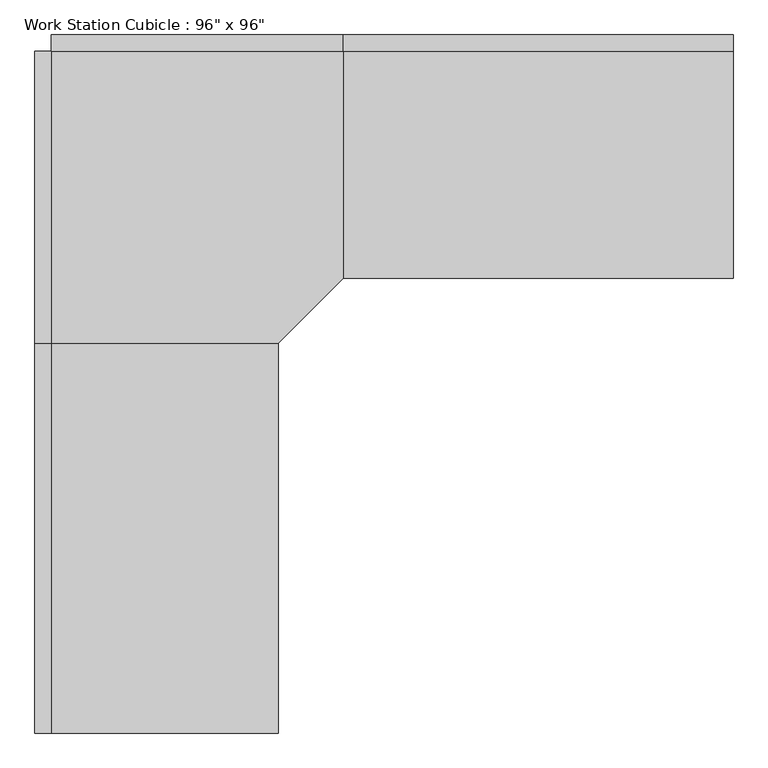
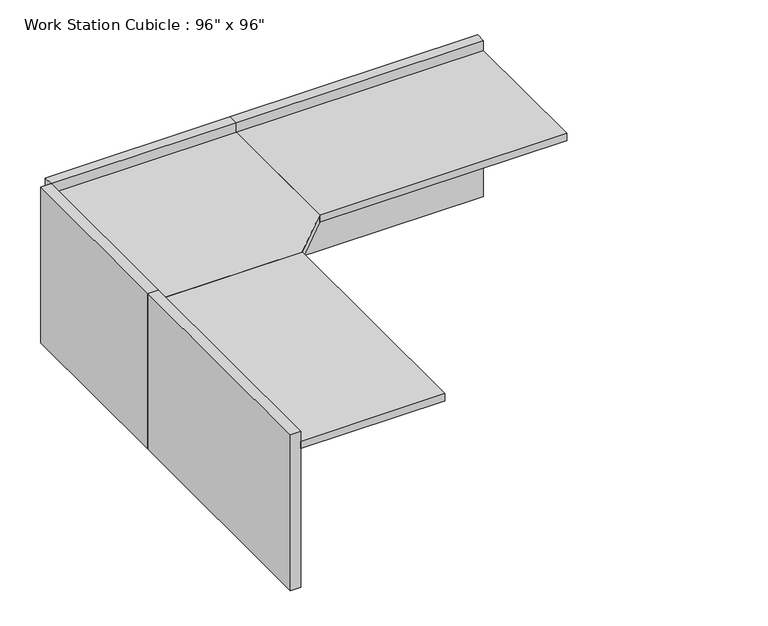
"""IFC4 building model written with IfcOpenShell, lengths in millimetres: furniture geometry."""

from ifc_helpers import new_model, si_unit, frame, origin, origin_with_axes, place, context, project, spatial, polyline, outline, extrude, source, transform, mapped, element, save


def furniture_65bc2ab2(model_context):
    return source(origin(), model_context, "Body", "SweptSolid", [
        extrude(outline(polyline([(-80.9317522, -545.8230076), (833.4682478, -545.8230076), (833.4682478, -1257.0230076), (630.2682478, -1460.2230076), (-80.9317522, -1460.2230076), (-80.9317522, -545.8230076)])), frame((0.0, 0.0, 723.9), z_axis=(0.0, 0.0, 1.0), x_axis=(1.0, 0.0, 0.0)), (0.0, 0.0, 1.0), 38.1),
        extrude(outline(polyline([(630.2682478, -2679.4230076), (-80.9317522, -2679.4230076), (-80.9317522, -1460.2230076), (630.2682478, -1460.2230076), (630.2682478, -2679.4230076)])), frame((0.0, 0.0, 723.9), z_axis=(0.0, 0.0, 1.0), x_axis=(1.0, 0.0, 0.0)), (0.0, 0.0, 1.0), 38.1),
        extrude(outline(polyline([(2052.6682478, -1257.0230076), (833.4682478, -1257.0230076), (833.4682478, -545.8230076), (2052.6682478, -545.8230076), (2052.6682478, -1257.0230076)])), frame((0.0, 0.0, 723.9), z_axis=(0.0, 0.0, 1.0), x_axis=(1.0, 0.0, 0.0)), (0.0, 0.0, 1.0), 38.1),
        extrude(outline(polyline([(2052.6682478, -545.8230076), (833.4682478, -545.8230076), (833.4682478, -495.0230076), (2052.6682478, -495.0230076), (2052.6682478, -545.8230076)])), origin_with_axes(), (0.0, 0.0, 1.0), 812.8),
        extrude(outline(polyline([(833.4682478, -545.8230076), (-80.9317522, -545.8230076), (-80.9317522, -495.0230076), (833.4682478, -495.0230076), (833.4682478, -545.8230076)])), origin_with_axes(), (0.0, 0.0, 1.0), 812.8),
        extrude(outline(polyline([(-80.9317522, -1460.2230076), (-131.7317522, -1460.2230076), (-131.7317522, -545.8230076), (-80.9317522, -545.8230076), (-80.9317522, -1460.2230076)])), origin_with_axes(), (0.0, 0.0, 1.0), 812.8),
        extrude(outline(polyline([(-80.9317522, -2679.4230076), (-131.7317522, -2679.4230076), (-131.7317522, -1460.2230076), (-80.9317522, -1460.2230076), (-80.9317522, -2679.4230076)])), origin_with_axes(), (0.0, 0.0, 1.0), 812.8),
    ])


if __name__ == "__main__":
    model = new_model("IFC4")
    model_context = context("Model", 3, world=origin())
    ifc_project = project(units=[si_unit("LENGTHUNIT", "METRE", prefix="MILLI")], contexts=[model_context])
    site = spatial("IfcSite", under=ifc_project)
    building = spatial("IfcBuilding", under=site)
    placement = place(None, origin())
    furniture_shape = furniture_65bc2ab2(model_context)
    element("IfcFurniture", 1, ObjectType="Work Station Cubicle : 96\" x 96\"", at=placement, inside=building, context=model_context, shape_type="MappedRepresentation", body=[
        mapped(furniture_shape, transform((0.0, 0.0, 0.0), x_axis=(1.0, 0.0, 0.0), y_axis=(0.0, 1.0, 0.0), z_axis=(0.0, 0.0, 1.0))),
    ])
    save(model, "model.ifc")

# Revit data of these elements
# Type "Work Station Cubicle : 96\" x 96\""
#   Assembly Code = "E2020"
#   Desktop Height = 2' - 6"
#   Desktop1 Width = 2' - 4"
#   Desktop2 Width = 2' - 4"
#   Panel Height = 2' - 8"
#   Panel1 Length = 4' - 0"
#   Panel2 Length = 4' - 0"
#   Cube Panel Material = Textile - Light Gray
#   Work Top Material = Laminate, Ivory, Matte
#   Default Elevation = 0
# Element 1 (IfcFurniture, "Work Station Cubicle : 96\" x 96\"")
#   Materials on its faces: "Textile - Light Gray", "Laminate, Ivory, Matte"
# Materials
#   "Textile - Light Gray": class "Fabric", colour RGB 204 204 204, transparency 0
#   "Laminate, Ivory, Matte": class "Plastic", colour RGB 247 247 239, transparency 0, Description = "Plastic Laminate - Ivory, Matte", Cost = 0
